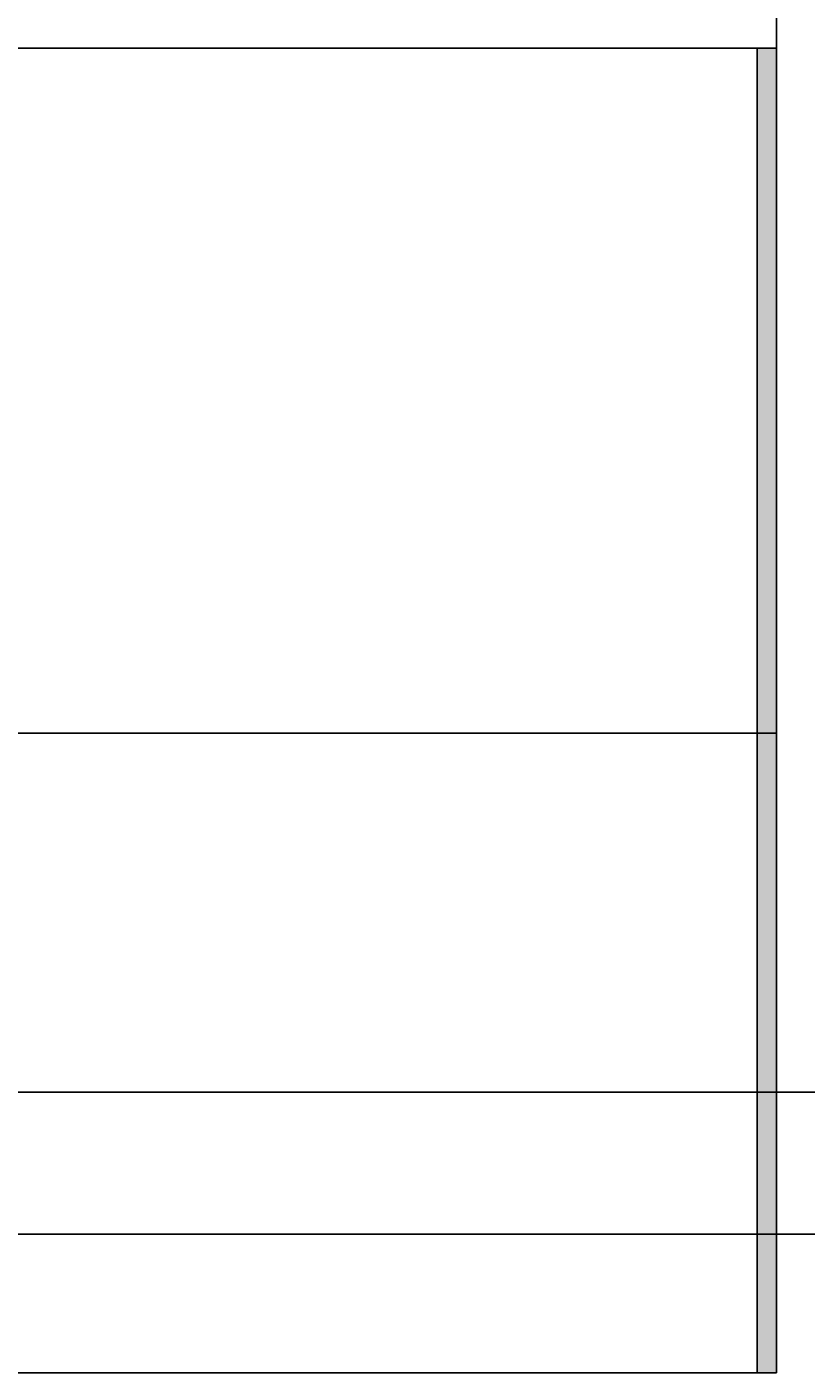
# Model space of a CAD drawing. Units: inches. Extents: x 35362 to 73946, y 43607 to 67532.
# Tile 88 of 134: x 51924 to 52380, y 47544 to 48331. Entities that reach past the tile are written whole.
import ezdxf

# ---------------------------------------------------------------- set-up
doc = ezdxf.new("R2010")
doc.units = ezdxf.units.IN
doc.header["$MEASUREMENT"] = 0
for name, color, linetype, lineweight in [('A-ANNO-DIMS', 2, 'Continuous', 18), ('E-SYMB', 1, 'Continuous', 25), ('E-SYMB-PATT', 1, 'Continuous', 13), ('E-WIRE', 3, 'Continuous', 25)]:
    doc.layers.add(name, color=color, linetype=linetype, lineweight=lineweight)
doc.styles.get("Standard").update_dxf_attribs({"font": 'arial.ttf'})
doc.dimstyles.get("Standard").update_dxf_attribs({"dimtxt": 0.18, "dimasz": 0.18, "dimexe": 0.18, "dimexo": 0.0625, "dimgap": 0.09, "dimtad": 0, "dimtih": 1, "dimtoh": 1, "dimdec": 4, "dimzin": 0, "dimdsep": 46, "dimtxsty": 'Standard', "dimcen": 0.09, "dimadec": 0, "dimazin": 0, "dimtfac": 1, "dimtdec": 4, "dimtofl": 0, "dimtmove": 0, "dimatfit": 3, "dimfxl": 1, "dimtolj": 1, "dimtzin": 0, "dimarcsym": 0})

# ---------------------------------------------------------------- blocks, each defined once
blk = doc.blocks.new('*D11')
at = {"layer": 'A-ANNO-DIMS', "color": 0, "lineweight": -2, "transparency": 16777216}
for p, q in [((47978.66, 56028.77), (47978.66, 43606.68)), ((53109.76, 56028.77), (53109.76, 43606.68)), ((47978.84, 43606.86), (50543.87, 43606.86)), ((53109.58, 43606.86), (50544.55, 43606.86))]:
    blk.add_line(p, q, dxfattribs=at)
at = {"layer": 'A-ANNO-DIMS', "color": 0, "transparency": 16777216}
for points in [[(47978.84, 43606.89), (47978.84, 43606.83), (47978.66, 43606.86)], [(53109.58, 43606.89), (53109.58, 43606.83), (53109.76, 43606.86)]]:
    blk.add_solid(points, dxfattribs=at)
at = {"layer": 'Defpoints', "color": 0, "transparency": 16777216}
for p in [(47978.66, 56028.84), (53109.76, 56028.84), (53109.76, 43606.86)]:
    blk.add_point(p, dxfattribs=at)
at = {"layer": 'A-ANNO-DIMS', "color": 0, "transparency": 16777216, "insert": (50544.21, 43606.86), "char_height": 0.18, "attachment_point": 5}
blk.add_mtext('\\A1;5131', dxfattribs=at)
blk = doc.blocks.new('*D43')
at = {"layer": 'A-ANNO-DIMS', "color": 0, "lineweight": -2, "transparency": 16777216}
for p, q in [((62004.67, 47625.18), (35361.77, 47625.18)), ((35361.95, 47625), (35361.95, 47416.9)), ((35361.95, 47208.43), (35361.95, 47416.53)), ((62004.67, 47208.25), (35361.77, 47208.25))]:
    blk.add_line(p, q, dxfattribs=at)
at = {"layer": 'A-ANNO-DIMS', "color": 0, "transparency": 16777216}
for points in [[(35361.92, 47625), (35361.98, 47625), (35361.95, 47625.18)], [(35361.92, 47208.43), (35361.98, 47208.43), (35361.95, 47208.25)]]:
    blk.add_solid(points, dxfattribs=at)
at = {"layer": 'Defpoints', "color": 0, "transparency": 16777216}
for p in [(62004.73, 47625.18), (35361.95, 47208.25), (62004.73, 47208.25)]:
    blk.add_point(p, dxfattribs=at)
at = {"layer": 'A-ANNO-DIMS', "color": 0, "transparency": 16777216, "insert": (35361.95, 47416.72), "char_height": 0.18, "attachment_point": 5}
blk.add_mtext('\\A1;416.9', dxfattribs=at)
blk = doc.blocks.new('*D67')
at = {"layer": 'A-ANNO-DIMS', "color": 0, "lineweight": -2, "transparency": 16777216}
for p, q in [((56873.54, 53351.53), (35361.77, 53351.53)), ((35361.95, 53351.35), (35361.95, 49400.89)), ((35361.95, 45450.07), (35361.95, 49400.53)), ((53793.58, 45449.89), (35361.77, 45449.89))]:
    blk.add_line(p, q, dxfattribs=at)
at = {"layer": 'A-ANNO-DIMS', "color": 0, "transparency": 16777216}
for points in [[(35361.92, 53351.35), (35361.98, 53351.35), (35361.95, 53351.53)], [(35361.92, 45450.07), (35361.98, 45450.07), (35361.95, 45449.89)]]:
    blk.add_solid(points, dxfattribs=at)
at = {"layer": 'Defpoints', "color": 0, "transparency": 16777216}
for p in [(35361.95, 53351.53), (56873.6, 53351.53), (53793.64, 45449.89)]:
    blk.add_point(p, dxfattribs=at)
at = {"layer": 'A-ANNO-DIMS', "color": 0, "transparency": 16777216, "insert": (35361.95, 49400.71), "char_height": 0.18, "attachment_point": 5}
blk.add_mtext('\\A1;7901.6', dxfattribs=at)
blk = doc.blocks.new('*D87')
at = {"layer": 'A-ANNO-DIMS', "color": 0, "lineweight": -2, "transparency": 16777216}
for p, q in [((52362.49, 48318.27), (35361.77, 48318.27)), ((35361.95, 48318.09), (35361.95, 47931.38)), ((35361.95, 47544.31), (35361.95, 47931.02)), ((52362.49, 47544.13), (35361.77, 47544.13))]:
    blk.add_line(p, q, dxfattribs=at)
at = {"layer": 'A-ANNO-DIMS', "color": 0, "transparency": 16777216}
for points in [[(35361.92, 48318.09), (35361.98, 48318.09), (35361.95, 48318.27)], [(35361.92, 47544.31), (35361.98, 47544.31), (35361.95, 47544.13)]]:
    blk.add_solid(points, dxfattribs=at)
at = {"layer": 'Defpoints', "color": 0, "transparency": 16777216}
for p in [(35361.95, 48318.27), (52362.56, 48318.27), (52362.56, 47544.13)]:
    blk.add_point(p, dxfattribs=at)
at = {"layer": 'A-ANNO-DIMS', "color": 0, "transparency": 16777216, "insert": (35361.95, 47931.2), "char_height": 0.18, "attachment_point": 5}
blk.add_mtext('\\A1;774.1', dxfattribs=at)
blk = doc.blocks.new('*D88')
at = {"layer": 'A-ANNO-DIMS', "color": 0, "lineweight": -2, "transparency": 16777216}
for p, q in [((52362.56, 48318.33), (52362.56, 67531.69)), ((52502.36, 48318.33), (52502.36, 67531.69)), ((52362.74, 67531.51), (52432.07, 67531.51)), ((52502.18, 67531.51), (52432.85, 67531.51))]:
    blk.add_line(p, q, dxfattribs=at)
at = {"layer": 'A-ANNO-DIMS', "color": 0, "transparency": 16777216}
for points in [[(52362.74, 67531.54), (52362.74, 67531.48), (52362.56, 67531.51)], [(52502.18, 67531.54), (52502.18, 67531.48), (52502.36, 67531.51)]]:
    blk.add_solid(points, dxfattribs=at)
at = {"layer": 'Defpoints', "color": 0, "transparency": 16777216}
for p in [(52502.36, 67531.51), (52362.56, 48318.27), (52502.36, 48318.27)]:
    blk.add_point(p, dxfattribs=at)
at = {"layer": 'A-ANNO-DIMS', "color": 0, "transparency": 16777216, "insert": (52432.46, 67531.51), "char_height": 0.18, "attachment_point": 5}
blk.add_mtext('\\A1;139.8', dxfattribs=at)
blk = doc.blocks.new('*D89')
at = {"layer": 'A-ANNO-DIMS', "color": 0, "lineweight": -2, "transparency": 16777216}
for p, q in [((53707.72, 48897.74), (35361.77, 48897.74)), ((35361.95, 48897.56), (35361.95, 48303.16)), ((35361.95, 47708.4), (35361.95, 48302.8)), ((53707.72, 47708.22), (35361.77, 47708.22))]:
    blk.add_line(p, q, dxfattribs=at)
at = {"layer": 'A-ANNO-DIMS', "color": 0, "transparency": 16777216}
for points in [[(35361.92, 48897.56), (35361.98, 48897.56), (35361.95, 48897.74)], [(35361.92, 47708.4), (35361.98, 47708.4), (35361.95, 47708.22)]]:
    blk.add_solid(points, dxfattribs=at)
at = {"layer": 'Defpoints', "color": 0, "transparency": 16777216}
for p in [(53707.78, 48897.74), (35361.95, 47708.22), (53707.78, 47708.22)]:
    blk.add_point(p, dxfattribs=at)
at = {"layer": 'A-ANNO-DIMS', "color": 0, "transparency": 16777216, "insert": (35361.95, 48302.98), "char_height": 0.18, "attachment_point": 5}
blk.add_mtext('\\A1;1189.5', dxfattribs=at)

msp = doc.modelspace()

# ---------------------------------------------------------------- hatches: boundary and pattern name
at = {"layer": 'E-SYMB-PATT'}
h = msp.add_hatch(color=256, dxfattribs=at)
h.dxf.hatch_style = 1
h.paths.add_polyline_path([(52351.402, 47544.134), (52362.557, 47544.134), (52362.557, 48318.269), (52351.402, 48318.269)])

# ---------------------------------------------------------------- linework, layer by layer
at = {"layer": 'E-SYMB'}
for p, q in [((52351.402, 48318.269), (52351.402, 47544.134)), ((52362.557, 47544.134), (52362.557, 48318.269)), ((52362.557, 47918.089), (52061.002, 47918.089)), ((52351.402, 47544.134), (52362.557, 47544.134))]:
    msp.add_line(p, q, dxfattribs=at)
at = {"layer": 'E-WIRE'}
msp.add_line((51540.551, 47918.089), (52061.002, 47918.089), dxfattribs=at)

# ---------------------------------------------------------------- dimensions: what is measured, and where the dimension line sits
at = {"layer": 'A-ANNO-DIMS'}
for base, p1, p2, override, picture, middle in [((52502.363, 67531.512), (52362.557, 48318.269), (52502.363, 48318.269), {"dimdec": 1, "dimlfac": 1, "dimrnd": 0, "dimzin": 0, "dimdsep": 46, "dimlunit": 2}, '*D88', (52432.46, 67531.512)), ((53109.76, 43606.859), (47978.665, 56028.836), (53109.76, 56028.836), {"dimdec": 0, "dimlfac": 1, "dimrnd": 0, "dimzin": 0, "dimdsep": 46, "dimlunit": 2}, '*D11', (50544.212, 43606.859))]:
    dim = msp.add_linear_dim(base=base, p1=p1, p2=p2, dimstyle='Standard', override=override, dxfattribs=at)
    dim.commit()
    dim.dimension.update_dxf_attribs({"geometry": picture, "text_midpoint": middle})
for base, p1, p2, picture, middle in [((35361.949, 53351.529), (53793.638, 45449.894), (56873.602, 53351.529), '*D67', (35361.949, 49400.712)), ((35361.949, 47708.216), (53707.781, 48897.738), (53707.781, 47708.216), '*D89', (35361.949, 48302.977)), ((35361.949, 48318.269), (52362.557, 47544.134), (52362.557, 48318.269), '*D87', (35361.949, 47931.201)), ((35361.949, 47208.25), (62004.728, 47625.181), (62004.728, 47208.25), '*D43', (35361.949, 47416.715))]:
    dim = msp.add_linear_dim(base=base, p1=p1, p2=p2, angle=90, dimstyle='Standard', override={"dimdec": 1, "dimlfac": 1, "dimrnd": 0, "dimzin": 0, "dimdsep": 46, "dimlunit": 2}, dxfattribs=at)
    dim.commit()
    dim.dimension.update_dxf_attribs({"geometry": picture, "text_midpoint": middle})

doc.saveas('drawing.dxf')
